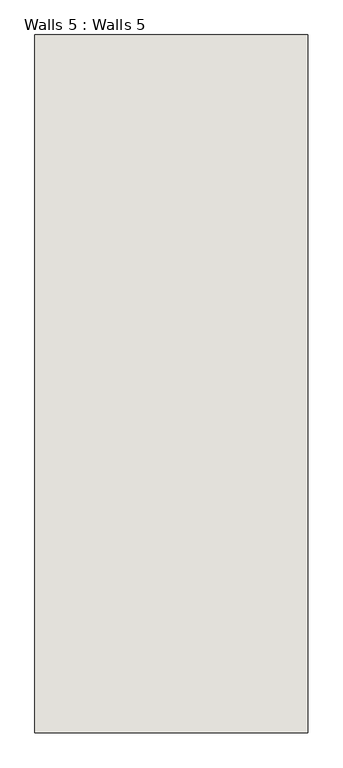
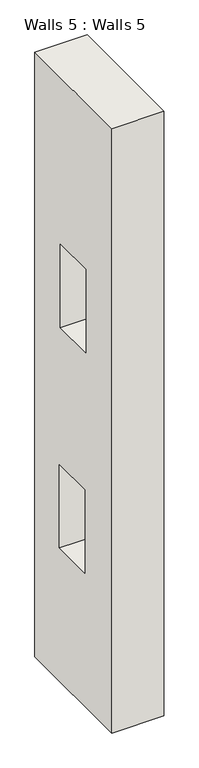
"""IFC4 building model written with IfcOpenShell, lengths in millimetres: wall geometry, Walls 5 : Walls 5."""

from ifc_helpers import new_model, si_unit, frame, origin, place, context, project, spatial, polyline, outline, extrude, source, transform, mapped, element, save


def walls_5_walls_5_33b50d55(model_context):
    return source(origin(), model_context, "Body", "SweptSolid", [
        extrude(outline(polyline([(7298.4643631, 3657.6), (7298.4643631, 12496.8), (9141.5373924, 12496.8), (9141.5373924, 3657.6), (7298.4643631, 3657.6)]), holes=[polyline([(8534.3701394, 8838.7474778), (8534.3701394, 10057.9474778), (7924.7701394, 10057.9474778), (7924.7701394, 8838.7474778), (8534.3701394, 8838.7474778)]), polyline([(8554.1972961, 5602.6860687), (8554.1972961, 6821.8860687), (7944.5972961, 6821.8860687), (7944.5972961, 5602.6860687), (8554.1972961, 5602.6860687)])]), frame((-10774.0916464, 0.0, 0.0), z_axis=(1.0, 0.0, 0.0), x_axis=(0.0, 1.0, 0.0)), (0.0, 0.0, 1.0), 720.6918992),
    ])


if __name__ == "__main__":
    model = new_model("IFC4")
    model_context = context("Model", 3, world=origin())
    ifc_project = project(units=[si_unit("LENGTHUNIT", "METRE", prefix="MILLI")], contexts=[model_context])
    site = spatial("IfcSite", under=ifc_project)
    building = spatial("IfcBuilding", under=site)
    placement = place(None, origin())
    walls_5_walls_5_shape = walls_5_walls_5_33b50d55(model_context)
    element("IfcWall", 1, ObjectType="Walls 5 : Walls 5", at=placement, inside=building, context=model_context, shape_type="MappedRepresentation", body=[
        mapped(walls_5_walls_5_shape, transform((0.0, 0.0, 0.0), x_axis=(1.0, 0.0, 0.0), y_axis=(0.0, 1.0, 0.0), z_axis=(0.0, 0.0, 1.0))),
    ])
    save(model, "model.ifc")

# Revit data of these elements
# Element 1 (IfcWall, "Walls 5 : Walls 5")
#   Materials on its faces: "Default Wall"
# Materials
#   "Default Wall": colour RGB 128 128 128, transparency 0
